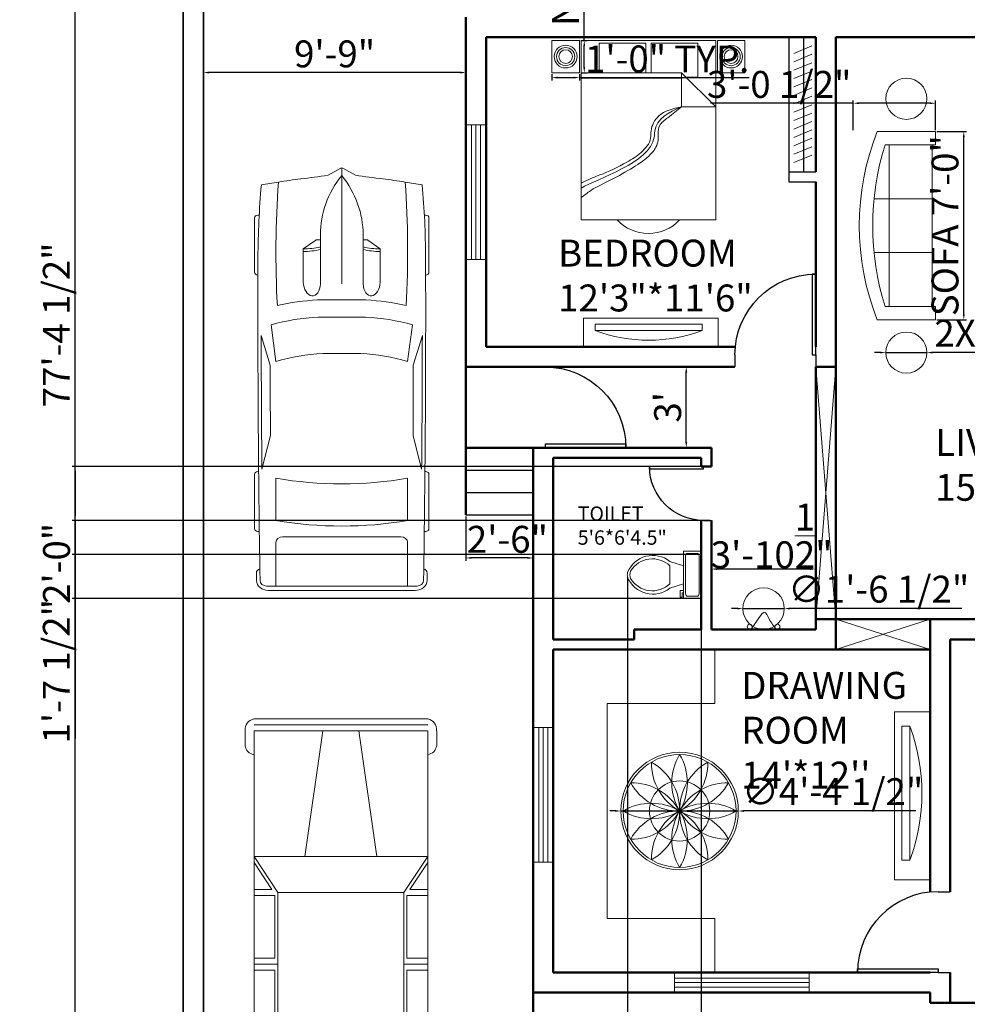
# Model space of a CAD drawing. Units: inches. Extents: x 6286 to 7213, y 5725 to 6776.
# Tile 2 of 5: x 6286 to 6709, y 5946 to 6385. Entities that reach past the tile are written whole.
import ezdxf

# ---------------------------------------------------------------- set-up
doc = ezdxf.new("R2010")
doc.units = ezdxf.units.IN
for name, color, linetype, lineweight in [('A-ANNO-DIMS', 2, 'Continuous', 18), ('A-AREA-IDEN', 7, 'Continuous', 25), ('A-DOOR', 3, 'Continuous', 25), ('A-FLOR-CASE', 8, 'Continuous', 25), ('A-FLOR-CASE-PATT', 252, 'Continuous', 13), ('A-FLOR-STRS', 7, 'Continuous', 25), ('A-FURN', 8, 'Continuous', 18), ('A-GLAZ', 4, 'Continuous', 18), ('A-WALL', 7, 'Continuous', 50), ('A-WALL-OPEN', 7, 'Continuous', 18), ('C-PKNG-VEHI', 8, 'Continuous', 13), ('C-PROP', 7, 'Continuous', 35), ('P-FLOR-FIXT', 9, 'Continuous', 18)]:
    doc.layers.add(name, color=color, linetype=linetype, lineweight=lineweight)
doc.styles.get("Standard").update_dxf_attribs({"font": 'arial.ttf'})
doc.dimstyles.new('ISO-25', dxfattribs={"dimtxt": 12, "dimasz": 2.5, "dimexe": 1.25, "dimexo": 0.625, "dimtad": 1, "dimdec": 1, "dimlunit": 4, "dimtxsty": 'Standard', "dimcen": 2.5, "dimadec": 0, "dimazin": 0, "dimtfac": 1, "dimtdec": 1, "dimtmove": 0, "dimatfit": 3, "dimfxl": 1, "dimarcsym": 0})

# ---------------------------------------------------------------- blocks, each defined once
blk = doc.blocks.new('*U2')
for p, q in [((0, 0), (0, -6)), ((40, 0), (40, -6))]:
    blk.add_line(p, q)
blk.add_lwpolyline([(0, 0), (0, 40), (1.75, 40), (1.75, 0)], close=True)
blk.add_arc((0, 0), 40, 0, 90)
blk = doc.blocks.new('*U10')
for p, q in [((9.5, -6), (9.5, -2)), ((-10, -8.5), (-8, -8.5)), ((-10, -9.5), (-10, -8.5)), ((-8, -8.5), (-8, -8)), ((-7, -8), (-7, -9.5)), ((-4, -8), (-6, -14)), ((4, -8), (6, -14)), ((-7, -9.5), (-10, -9.5)), ((4, -14), (-4, -14))]:
    blk.add_line(p, q)
blk.add_lwpolyline([(10.5, -8), (10.5, 0), (-10.5, 0), (-10.5, -8)], close=True)
for points in [[(-9.5, -2), (-9.5, -6)], [(8.5, -1), (-8.5, -1)], [(-8.5, -7), (8.5, -7)]]:
    blk.add_lwpolyline(points)
for centre, radius, start, end in [((-8.62, -1.88), 0.884, 81.8699, 188.1301), ((8.62, -1.88), 0.884, 351.8699, 98.1301), ((-8.62, -6.12), 0.884, 171.8699, 278.1301), ((8.62, -6.12), 0.884, 261.8699, 8.1301), ((3.52, -21.58), 12.17, 141.4691, 247.9714), ((4.2, -21.82), 11.33, 136.3677, 238.9468), ((-3.52, -21.58), 12.17, 292.0284, 38.5307), ((-4.2, -21.82), 11.33, 301.053, 43.6321), ((0, -27.88), 4, 245.7318, 294.2682), ((0, -29), 4, 254.8605, 285.1395)]:
    blk.add_arc(centre, radius, start, end)
blk = doc.blocks.new('Sofa - Roundback 7 ft.')
for p, q in [((-12.00002, -32.4421), (-12.00003, -6.5971)), ((11.99997, -32.4421), (11.99998, -6.5971)), ((-36.000027, -34), (-36.000027, -11.4696)), ((35.99998, -34), (35.99998, -11.4696)), ((-35.999844, -13.3819), (35.9998, -13.3819)), ((-36.000027, -32.4421), (35.99998, -32.4421))]:
    blk.add_line(p, q)
for points in [[(-36.000027, -34), (-42.000027, -34), (-42.000027, -8)], [(41.99998, -8), (41.99998, -34), (35.99998, -34)]]:
    blk.add_lwpolyline(points)
for centre, radius, start, end in [((0, -114.25), 114.25, 68.43141, 111.5686), ((-0.00001, -127.1968), 121.1968, 72.72033, 107.2797)]:
    blk.add_arc(centre, radius, start, end)
blk = doc.blocks.new('*D13')
at = {"layer": 'A-ANNO-DIMS', "color": 0, "lineweight": -2, "transparency": 16777216}
for p, q in [((6593.8, 6230.26), (6581.95, 6230.26)), ((6583.2, 6196.76), (6583.2, 6227.76)), ((6593.8, 6194.26), (6581.95, 6194.26))]:
    blk.add_line(p, q, dxfattribs=at)
at = {"layer": 'A-ANNO-DIMS', "color": 0, "lineweight": 100, "transparency": 16777216}
for points in [[(6582.79, 6227.76), (6583.62, 6227.76), (6583.2, 6230.26)], [(6582.79, 6196.76), (6583.62, 6196.76), (6583.2, 6194.26)]]:
    blk.add_solid(points, dxfattribs=at)
at = {"layer": 'Defpoints', "color": 0, "lineweight": 100, "transparency": 16777216}
for p in [(6583.2, 6230.26), (6594.42, 6230.26), (6594.42, 6194.26)]:
    blk.add_point(p, dxfattribs=at)
at = {"layer": 'A-ANNO-DIMS', "color": 0, "transparency": 16777216, "insert": (6576.45, 6212.26), "char_height": 12, "attachment_point": 5, "rotation": 90}
blk.add_mtext("3'", dxfattribs=at)
blk = doc.blocks.new('*D14')
at = {"layer": 'A-ANNO-DIMS', "color": 0, "lineweight": -2, "transparency": 16777216}
for p, q in [((6484.92, 6163.64), (6484.92, 6143.83)), ((6514.92, 6163.64), (6514.92, 6143.83)), ((6512.42, 6145.08), (6487.42, 6145.08))]:
    blk.add_line(p, q, dxfattribs=at)
at = {"layer": 'A-ANNO-DIMS', "color": 0, "lineweight": 100, "transparency": 16777216}
for points in [[(6487.42, 6145.5), (6487.42, 6144.67), (6484.92, 6145.08)], [(6512.42, 6145.5), (6512.42, 6144.67), (6514.92, 6145.08)]]:
    blk.add_solid(points, dxfattribs=at)
at = {"layer": 'Defpoints', "color": 0, "lineweight": 100, "transparency": 16777216}
for p in [(6484.92, 6164.26), (6514.92, 6164.26), (6484.92, 6145.08)]:
    blk.add_point(p, dxfattribs=at)
at = {"layer": 'A-ANNO-DIMS', "color": 0, "transparency": 16777216, "insert": (6503.46, 6151.84), "char_height": 12, "attachment_point": 5}
blk.add_mtext('2\'-6"', dxfattribs=at)
blk = doc.blocks.new('*D15')
at = {"layer": 'A-ANNO-DIMS', "color": 0, "lineweight": -2, "transparency": 16777216}
for p, q in [((6594.42, 6113.89), (6594.42, 6141.38)), ((6638.42, 6140.13), (6596.92, 6140.13)), ((6640.92, 6113.89), (6640.92, 6141.38))]:
    blk.add_line(p, q, dxfattribs=at)
at = {"layer": 'A-ANNO-DIMS', "color": 0, "lineweight": 100, "transparency": 16777216}
for points in [[(6596.92, 6140.55), (6596.92, 6139.71), (6594.42, 6140.13)], [(6638.42, 6140.55), (6638.42, 6139.71), (6640.92, 6140.13)]]:
    blk.add_solid(points, dxfattribs=at)
at = {"layer": 'Defpoints', "color": 0, "lineweight": 100, "transparency": 16777216}
for p in [(6594.42, 6140.13), (6594.42, 6113.26), (6640.92, 6113.26)]:
    blk.add_point(p, dxfattribs=at)
at = {"layer": 'A-ANNO-DIMS', "color": 0, "transparency": 16777216, "insert": (6621.27, 6154.91), "char_height": 12, "attachment_point": 5}
blk.add_mtext('3\'-10{\\H1x;\\S1/2;}"', dxfattribs=at)
blk = doc.blocks.new('*D25')
at = {"layer": 'A-ANNO-DIMS', "color": 0, "lineweight": -2, "transparency": 16777216}
for p, q in [((6367.92, 6385.64), (6367.92, 6360.28)), ((6484.92, 6385.64), (6484.92, 6360.28)), ((6482.42, 6361.53), (6370.42, 6361.53))]:
    blk.add_line(p, q, dxfattribs=at)
at = {"layer": 'A-ANNO-DIMS', "color": 0, "lineweight": 100, "transparency": 16777216}
for points in [[(6370.42, 6361.95), (6370.42, 6361.12), (6367.92, 6361.53)], [(6482.42, 6361.95), (6482.42, 6361.12), (6484.92, 6361.53)]]:
    blk.add_solid(points, dxfattribs=at)
at = {"layer": 'Defpoints', "color": 0, "lineweight": 100, "transparency": 16777216}
for p in [(6367.92, 6386.26), (6484.92, 6386.26), (6367.92, 6361.53)]:
    blk.add_point(p, dxfattribs=at)
at = {"layer": 'A-ANNO-DIMS', "color": 0, "transparency": 16777216, "insert": (6426.42, 6368.29), "char_height": 12, "attachment_point": 5}
blk.add_mtext('9\'-9"', dxfattribs=at)
blk = doc.blocks.new('*U27')
for p, q in [((21.1, 37.41), (21.1, 36.83)), ((46.55, 38.89), (22.35, 38.89)), ((47.8, 37.39), (47.8, 37.41)), ((87.99, 31.87), (74.76, 35.92)), ((134.31, 35.6), (119.29, 31.78)), ((135.45, 37.07), (135.45, 37.41)), ((136.7, 38.89), (160.9, 38.89)), ((162.15, 37.41), (162.15, 36.77)), ((70.03, 31.54), (86.41, 29.35)), ((186.47, -33.5), (186.47, 33.5)), ((188.4, -32.76), (188.4, 32.76)), ((138.42, 29.35), (157.25, 29.35)), ((164.52, 26.39), (164.52, -26.39)), ((186.47, 29.35), (167.01, 29.35)), ((32.27, 11.63), (36.13, 17.17)), ((36.13, 17.17), (50.94, 17.17)), ((29.77, 9.51), (51.68, 9.51)), ((32.12, 9.51), (32.12, 11.15)), ((58.92, -10.77), (58.92, 10.77)), ((66.55, -10.53), (66.55, 10.53)), ((186.47, -10.53), (186.47, 10.53)), ((3.27, 6.13), (0.1, 0.41)), ((82.74, 8.5), (82.74, -8.5)), ((0, 0), (51.68, 0)), ((0.1, -0.41), (3.27, -6.13)), ((29.77, -9.51), (51.68, -9.51)), ((32.12, -9.51), (32.12, -11.15)), ((32.27, -11.63), (36.13, -17.17)), ((36.13, -17.17), (50.94, -17.17)), ((86.41, -29.35), (70.03, -31.54)), ((157.25, -29.35), (138.42, -29.35)), ((167.01, -29.35), (186.47, -29.35)), ((87.99, -31.87), (74.76, -35.92)), ((134.31, -35.6), (119.29, -31.78)), ((21.1, -37.41), (21.1, -36.83)), ((46.55, -38.89), (22.35, -38.89)), ((47.8, -37.39), (47.8, -37.41)), ((135.45, -37.07), (135.45, -37.41)), ((136.7, -38.89), (160.9, -38.89)), ((162.15, -37.41), (162.15, -36.77))]:
    blk.add_line(p, q)
for centre, major_axis, ratio, start_param, end_param in [((266.03, -27.52), (0, 313.31), 0.842304, 1.367076, 1.39176), ((41.19, -490.86), (0, 528.23), 0.842304, 0.00281, 0.075598), ((22.35, 37.41), (0, -1.48), 0.842304, 3.141593, 4.712389), ((64.48, -10555.62), (0, 10593.03), 0.842304, -0.013397, 0.002797), ((46.55, 37.41), (0, 1.48), 0.842304, -1.570796, 0), ((64.48, -10555.62), (0, -10591.55), 0.842304, 3.133765, 3.140441), ((136.7, 37.41), (0, -1.48), 0.842304, 3.141593, 4.712389), ((160.9, 37.41), (0, 1.48), 0.842304, -1.570796, 0), ((180.63, 35.84), (0, 2.22), 0.842304, -0.013017, 1.249894), ((64.48, -10556.36), (0, 10595.31), 0.842304, -0.013397, -0.013017), ((183.98, 33.5), (0, -2.96), 0.842304, 1.570796, 3.128196), ((183.98, 32.76), (0, -5.25), 0.842304, 1.570796, 3.128196), ((135.29, 5.39), (0, 81.77), 0.842304, 1.245306, 1.50788), ((95.79, -3666.35), (0, -3698.24), 0.842304, 3.134049, 3.144098), ((259.18, -27.52), (0, -305.3), 0.842304, 4.528606, 4.561838), ((37.47, -593.96), (0, -623.33), 0.842304, 3.096046, 3.200911), ((134.4, 5.39), (0, -89.78), 0.842304, 4.449482, 4.652344), ((149.6, 2.8), (0, -79.58), 0.842304, 4.372215, 4.640744), ((17.08, 0), (0, 147.02), 0.842304, 4.511394, 4.913384), ((35.91, 0), (0, 147.02), 0.842304, 4.511394, 4.913384), ((167.01, 26.39), (0, 2.96), 0.842304, 0, 1.570796), ((-204.49, 52.4), (0, -250.96), 0.842304, 1.385369, 1.434372), ((13.04, 17.01), (0, 27.42), 0.842304, 4.435146, 4.718221), ((14.2, 17.01), (0, 27.42), 0.842304, 4.435146, 4.718221), ((50.79, 13.34), (6.34, -0.36), 0.603834, -1.395552, 1.581315), ((29.77, -46.66), (0, 56.17), 0.842304, 0, 0.590319), ((32.75, 11.15), (0, 0.74), 0.842304, 0.879714, 1.570796), ((0.62, 0), (0, -0.74), 0.842304, 4.131459, 5.293319), ((29.77, 46.66), (0, 56.17), 0.842304, 2.551274, 3.141593), ((-204.49, -52.4), (0, 250.96), 0.842304, -1.434372, -1.385369), ((149.6, -2.8), (0, -79.58), 0.842304, -1.499151, -1.230623), ((32.75, -11.15), (0, -0.74), 0.842304, 4.712389, 5.403472), ((13.04, -17.01), (0, -27.42), 0.842304, 1.564964, 1.848039), ((14.2, -17.01), (0, -27.42), 0.842304, 1.564964, 1.848039), ((134.4, -5.39), (0, -89.78), 0.842304, -1.510751, -1.307889), ((135.29, -5.39), (0, -81.77), 0.842304, -1.50788, -1.245306), ((259.18, 27.52), (0, 305.3), 0.842304, 1.721348, 1.754579), ((266.03, 27.52), (0, 313.31), 0.842304, 1.749832, 1.774517), ((37.47, 593.96), (0, -623.33), 0.842304, -0.059319, 0.045547), ((167.01, -26.39), (0, -2.96), 0.842304, 4.712389, 6.283185), ((95.79, 3666.35), (0, -3698.24), 0.842304, -0.002505, 0.007544), ((183.98, -33.5), (0, 2.96), 0.842304, 3.15499, 4.712389), ((183.98, -32.76), (0, -5.25), 0.842304, 0.013397, 1.570796), ((41.19, 490.86), (0, -528.23), 0.842304, -0.075598, -0.00281), ((22.35, -37.41), (0, 1.48), 0.842304, 1.570796, 3.141593), ((64.48, 10555.62), (0, 10593.03), 0.842304, 3.138796, 3.15499), ((46.55, -37.41), (0, -1.48), 0.842304, 0, 1.570796), ((64.48, 10555.62), (0, -10591.55), 0.842304, 0.001152, 0.007828), ((136.7, -37.41), (0, -1.48), 0.842304, -1.570796, 0), ((160.9, -37.41), (0, 1.48), 0.842304, 3.141593, 4.712389), ((180.63, -35.84), (0, -2.22), 0.842304, -1.249894, 0.013017), ((64.48, 10556.36), (0, 10595.31), 0.842304, 3.15461, 3.15499)]:
    blk.add_ellipse(centre, major_axis=major_axis, ratio=ratio, start_param=start_param, end_param=end_param)
at = {"extrusion": (0, 0, -1)}
blk.add_ellipse((50.79, -13.34), major_axis=(6.34, 0.36), ratio=0.603834, start_param=-1.395552, end_param=1.581315, dxfattribs=at)
blk = doc.blocks.new('*U28')
for p, q in [((5.44, 42.31), (12.12, 42.31)), ((189.69, 42.31), (183.01, 42.31)), ((0.1, -0.41), (0.1, 38.35)), ((2.77, -0.41), (2.77, 38.31)), ((5.44, -0.41), (5.44, 38.24)), ((5.45, 38.31), (16.12, 38.31)), ((16.12, 38.31), (180.34, 38.31)), ((61.52, -0.41), (61.52, 38.31)), ((61.52, 38.31), (77.54, 27.62)), ((64.19, 38.31), (76.2, 30.29)), ((76.2, 30.29), (76.2, 38.31)), ((78.87, 38.31), (78.87, 28.96)), ((106.91, 28.96), (106.91, 38.31)), ((109.58, 27.62), (109.58, 38.31)), ((112.25, 38.31), (112.25, 28.96)), ((140.29, 28.96), (140.29, 38.31)), ((141.62, 27.62), (149.64, 38.31)), ((149.64, -0.41), (149.64, 38.31)), ((189.69, 38.31), (179.01, 38.31)), ((189.69, -0.41), (189.69, 38.24)), ((192.36, -0.41), (192.36, 38.31)), ((195.03, -0.41), (195.03, 38.35)), ((77.54, 27.62), (141.62, 27.62)), ((77.54, -0.41), (77.54, 27.62)), ((78.87, 28.96), (106.91, 28.96)), ((112.25, 28.96), (140.29, 28.96)), ((141.62, -0.41), (141.62, 27.62)), ((5.44, 7.6), (61.52, 15.61)), ((0.1, -0.42), (0.1, -39.18)), ((2.77, -0.41), (2.77, -39.13)), ((5.44, -0.42), (5.44, -39.07)), ((61.52, -0.41), (61.52, -39.13)), ((77.54, -0.41), (77.54, -28.45)), ((141.62, -0.41), (141.62, -28.45)), ((149.64, -0.41), (149.64, -39.13)), ((189.69, -0.42), (189.69, -39.07)), ((192.36, -0.41), (192.36, -39.13)), ((195.03, -0.42), (195.03, -39.18)), ((5.44, -8.42), (61.52, -16.43)), ((61.52, -39.13), (77.54, -28.45)), ((77.54, -28.45), (141.62, -28.45)), ((78.87, -39.13), (78.87, -29.79)), ((78.87, -29.79), (106.91, -29.79)), ((106.91, -29.79), (106.91, -39.13)), ((109.58, -28.45), (109.58, -39.13)), ((112.25, -29.79), (140.29, -29.79)), ((112.25, -39.13), (112.25, -29.79)), ((140.29, -29.79), (140.29, -39.13)), ((141.62, -28.45), (149.64, -39.13)), ((64.19, -39.13), (76.2, -31.12)), ((76.2, -31.12), (76.2, -39.13)), ((5.45, -39.13), (16.12, -39.13)), ((16.12, -39.13), (180.34, -39.13)), ((189.69, -39.13), (179.01, -39.13)), ((5.44, -43.14), (12.12, -43.14)), ((189.69, -43.14), (183.01, -43.14))]:
    blk.add_line(p, q)
for centre, radius, start, end in [((5.06, 37.26), 5.06, 85.6455, 168.0943), ((11.45, 37.64), 4.72, 8.1301, 81.87), ((183.68, 37.64), 4.72, 98.13, 171.8699), ((190.07, 37.26), 5.06, 11.9057, 94.3545), ((5.06, -38.09), 5.06, 191.9057, 274.3545), ((11.45, -38.46), 4.72, 278.13, 351.8699), ((183.68, -38.46), 4.72, 188.1301, 261.87), ((190.07, -38.09), 5.06, 265.6455, 348.0943)]:
    blk.add_arc(centre, radius, start, end)
blk = doc.blocks.new('WIN-60IN')
for p, q in [((0, 9), (0, 0)), ((60, 0), (60, 9)), ((60, 6.5), (0, 6.5)), ((60, 4.5), (0, 4.5)), ((60, 2.5), (0, 2.5))]:
    blk.add_line(p, q)
blk = doc.blocks.new('NIGHTSTAND-LAMP')
blk.add_lwpolyline([(12.23, 14.4), (0, 14.4), (0, 0), (12.23, 0)], close=True)
for radius in [5.06, 4.06, 3.06]:
    blk.add_circle((6.12, 7.2), radius)
blk = doc.blocks.new('TV-CONSOLE-60IN')
for points in [[(0, 12.71), (60, 12.71), (60, 0), (0, 0)], [(5.19, 10.13), (52.94, 10.13), (52.94, 7.18), (5.19, 7.18)]]:
    blk.add_lwpolyline(points, close=True)
blk.add_arc((29.07, 71.71), 68.81, 249.6947, 290.3053)
blk = doc.blocks.new('Bed - Queen')
for p, q in [((0, -80.00003), (0, 0)), ((0, 0), (59.99999, 0)), ((59.99999, 0), (59.99999, -80.00003)), ((7.99999, -1.2), (28.79998, -1.2)), ((7.99999, -14.4), (7.99999, -1.2)), ((28.79998, -1.2), (28.79998, -14.4)), ((31.19999, -1.2), (51.99999, -1.2)), ((31.19999, -14.4), (31.19999, -1.2)), ((51.99999, -1.2), (51.99999, -16.4)), ((0, -14.4), (44.8, -14.4)), ((44.8, -16.8), (0, -16.8)), ((59.99999, -29.6), (44.8, -14.4)), ((44.8, -14.4), (44.8, -29.6)), ((51.99999, -16.4), (46.79936, -16.4)), ((44.8, -29.6), (59.99999, -29.6)), ((59.99999, -80.00003), (0, -80.00003))]:
    blk.add_line(p, q)
blk = doc.blocks.new('BED-QUEEN-DRESSED')
blk.add_arc((30, 18.96), 18.96, 222.7518, 317.2482)
for points, knots in [([(44.8, 56.49), (39.19, 53.96), (32.77, 51.07), (32.71, 32.08), (7.2, 24.53), (0, 20.27)], [0, 0, 0, 0, 16.08431, 18.417841, 48.068097, 48.068097, 48.068097, 48.068097]), ([(44.8, 56.49), (41.02, 55.65), (34.77, 54.26), (30.9, 47.2), (31.38, 41.03), (26.76, 35.63), (19.36, 31.03), (9.68, 26.38), (4.48, 24.69), (0, 22.46)], [0, 0, 0, 0, 11.066231, 18.341473, 21.645482, 29.256421, 37.126455, 49.94498, 57.001864, 57.001864, 57.001864, 57.001864]), ([(44.8, 56.49), (42.82, 54.88), (39.55, 52.2), (33.5, 47.94), (35.23, 40.79), (30.55, 34.13), (23.14, 29.37), (13.11, 23.54), (6.2, 20.75), (1.43, 17.09), (0, 16.03)], [0, 0, 0, 0, 7.83924, 12.978287, 20.287315, 26.568624, 36.127852, 46.548326, 57.45004, 62.118815, 62.118815, 62.118815, 62.118815])]:
    blk.add_open_spline(points, degree=3, knots=knots)
blk.add_blockref('Bed - Queen', (0, 86.09))
blk = doc.blocks.new('WARDROBE-RETURN-RAIL')
for p, q in [((0, 64.5), (0, 0)), ((6.49, 64.5), (6.49, 4.5)), ((0, 4.5), (12, 4.5)), ((0, 0), (12, 0))]:
    blk.add_line(p, q)
blk = doc.blocks.new('*D43')
at = {"layer": 'A-ANNO-DIMS', "color": 0, "lineweight": -2, "transparency": 16777216}
for p, q in [((6537.72, 6375.84), (6537.72, 6593.74)), ((6536.18, 6375.84), (6538.97, 6375.84)), ((6537.72, 6363.94), (6537.72, 6373.34)), ((6536.18, 6361.44), (6538.97, 6361.44))]:
    blk.add_line(p, q, dxfattribs=at)
at = {"layer": 'A-ANNO-DIMS', "color": 0, "lineweight": 100, "transparency": 16777216}
for points in [[(6537.3, 6373.34), (6538.13, 6373.34), (6537.72, 6375.84)], [(6537.3, 6363.94), (6538.13, 6363.94), (6537.72, 6361.44)]]:
    blk.add_solid(points, dxfattribs=at)
at = {"layer": 'Defpoints', "color": 0, "lineweight": 100, "transparency": 16777216}
for p in [(6535.56, 6375.84), (6537.72, 6375.84), (6535.56, 6361.44)]:
    blk.add_point(p, dxfattribs=at)
at = {"layer": 'A-ANNO-DIMS', "color": 0, "transparency": 16777216, "insert": (6530.89, 6486.04), "char_height": 12, "attachment_point": 5, "rotation": 90}
blk.add_mtext('NIGHTSTAND 1\'-2 1/2" TYP.', dxfattribs=at)
blk = doc.blocks.new('*D44')
at = {"layer": 'A-ANNO-DIMS', "color": 0, "lineweight": -2, "transparency": 16777216}
for p, q in [((6523.32, 6360.81), (6523.32, 6358.03)), ((6525.82, 6359.28), (6533.06, 6359.28)), ((6535.56, 6360.81), (6535.56, 6358.03)), ((6535.56, 6359.28), (6611.32, 6359.28))]:
    blk.add_line(p, q, dxfattribs=at)
at = {"layer": 'A-ANNO-DIMS', "color": 0, "lineweight": 100, "transparency": 16777216}
for points in [[(6525.82, 6359.69), (6525.82, 6358.86), (6523.32, 6359.28)], [(6533.06, 6359.69), (6533.06, 6358.86), (6535.56, 6359.28)]]:
    blk.add_solid(points, dxfattribs=at)
at = {"layer": 'Defpoints', "color": 0, "lineweight": 100, "transparency": 16777216}
for p in [(6523.32, 6361.44), (6535.56, 6361.44), (6535.56, 6359.28)]:
    blk.add_point(p, dxfattribs=at)
at = {"layer": 'A-ANNO-DIMS', "color": 0, "transparency": 16777216, "insert": (6574.69, 6366.03), "char_height": 12, "attachment_point": 5}
blk.add_mtext('1\'-0" TYP.', dxfattribs=at)
blk = doc.blocks.new('*D53')
at = {"layer": 'A-ANNO-DIMS', "color": 0, "lineweight": -2, "transparency": 16777216}
for p, q in [((6694.98, 6335.25), (6708.2, 6335.25)), ((6706.95, 6253.75), (6706.95, 6332.75)), ((6694.98, 6251.25), (6708.2, 6251.25))]:
    blk.add_line(p, q, dxfattribs=at)
at = {"layer": 'A-ANNO-DIMS', "color": 0, "lineweight": 100, "transparency": 16777216}
for points in [[(6706.54, 6332.75), (6707.37, 6332.75), (6706.95, 6335.25)], [(6706.54, 6253.75), (6707.37, 6253.75), (6706.95, 6251.25)]]:
    blk.add_solid(points, dxfattribs=at)
at = {"layer": 'Defpoints', "color": 0, "lineweight": 100, "transparency": 16777216}
for p in [(6694.35, 6335.25), (6706.95, 6335.25), (6694.35, 6251.25)]:
    blk.add_point(p, dxfattribs=at)
at = {"layer": 'A-ANNO-DIMS', "color": 0, "transparency": 16777216, "insert": (6700.12, 6293.25), "char_height": 12, "attachment_point": 5, "rotation": 90}
blk.add_mtext('SOFA 7\'-0"', dxfattribs=at)
blk = doc.blocks.new('*D54')
at = {"layer": 'A-ANNO-DIMS', "color": 0, "lineweight": -2, "transparency": 16777216}
for p, q in [((6657.69, 6335.87), (6657.69, 6349.1)), ((6694.35, 6335.87), (6694.35, 6349.1)), ((6657.69, 6347.85), (6594.08, 6347.85)), ((6691.85, 6347.85), (6660.19, 6347.85))]:
    blk.add_line(p, q, dxfattribs=at)
at = {"layer": 'A-ANNO-DIMS', "color": 0, "lineweight": 100, "transparency": 16777216}
for points in [[(6660.19, 6348.26), (6660.19, 6347.43), (6657.69, 6347.85)], [(6691.85, 6348.26), (6691.85, 6347.43), (6694.35, 6347.85)]]:
    blk.add_solid(points, dxfattribs=at)
at = {"layer": 'Defpoints', "color": 0, "lineweight": 100, "transparency": 16777216}
for p in [(6657.69, 6347.85), (6657.69, 6335.25), (6694.35, 6335.25)]:
    blk.add_point(p, dxfattribs=at)
at = {"layer": 'A-ANNO-DIMS', "color": 0, "transparency": 16777216, "insert": (6624.64, 6354.68), "char_height": 12, "attachment_point": 5}
blk.add_mtext('3\'-0 1/2"', dxfattribs=at)
blk = doc.blocks.new('*D56')
at = {"layer": 'A-ANNO-DIMS', "color": 0, "lineweight": -2, "transparency": 16777216}
for p, q in [((6358.3, 6713.26), (6309.47, 6713.26)), ((6310.72, 5787.26), (6310.72, 6710.76)), ((6358.3, 5784.76), (6309.47, 5784.76))]:
    blk.add_line(p, q, dxfattribs=at)
at = {"layer": 'A-ANNO-DIMS', "color": 0, "lineweight": 100, "transparency": 16777216}
for points in [[(6310.31, 6710.76), (6311.14, 6710.76), (6310.72, 6713.26)], [(6310.31, 5787.26), (6311.14, 5787.26), (6310.72, 5784.76)]]:
    blk.add_solid(points, dxfattribs=at)
at = {"layer": 'Defpoints', "color": 0, "lineweight": 100, "transparency": 16777216}
for p in [(6310.72, 6713.26), (6358.92, 6713.26), (6358.92, 5784.76)]:
    blk.add_point(p, dxfattribs=at)
at = {"layer": 'A-ANNO-DIMS', "color": 0, "transparency": 16777216, "insert": (6303.89, 6249.01), "char_height": 12, "attachment_point": 5, "rotation": 90}
blk.add_mtext('77\'-4 1/2"', dxfattribs=at)
blk = doc.blocks.new('*D68')
at = {"layer": 'A-ANNO-DIMS', "color": 0, "lineweight": -2, "transparency": 16777216}
for p, q in [((6593.8, 6185.85), (6309.47, 6185.85)), ((6310.72, 6183.35), (6310.72, 6164.35)), ((6593.8, 6161.85), (6309.47, 6161.85)), ((6310.72, 6161.85), (6310.72, 6126))]:
    blk.add_line(p, q, dxfattribs=at)
at = {"layer": 'A-ANNO-DIMS', "color": 0, "lineweight": 100, "transparency": 16777216}
for points in [[(6310.31, 6183.35), (6311.14, 6183.35), (6310.72, 6185.85)], [(6310.31, 6164.35), (6311.14, 6164.35), (6310.72, 6161.85)]]:
    blk.add_solid(points, dxfattribs=at)
at = {"layer": 'Defpoints', "color": 0, "lineweight": 100, "transparency": 16777216}
for p in [(6594.42, 6185.85), (6310.72, 6161.85), (6594.42, 6161.85)]:
    blk.add_point(p, dxfattribs=at)
at = {"layer": 'A-ANNO-DIMS', "color": 0, "transparency": 16777216, "insert": (6303.97, 6142.67), "char_height": 12, "attachment_point": 5, "rotation": 90}
blk.add_mtext('2\'-0"', dxfattribs=at)
blk = doc.blocks.new('*D69')
at = {"layer": 'A-ANNO-DIMS', "color": 0, "lineweight": -2, "transparency": 16777216}
for p, q in [((6589.3, 6146.57), (6309.47, 6146.57)), ((6310.72, 6144.07), (6310.72, 6129.57)), ((6589.3, 6127.07), (6309.47, 6127.07)), ((6310.72, 6127.07), (6310.72, 6064.58))]:
    blk.add_line(p, q, dxfattribs=at)
at = {"layer": 'A-ANNO-DIMS', "color": 0, "lineweight": 100, "transparency": 16777216}
for points in [[(6310.31, 6144.07), (6311.14, 6144.07), (6310.72, 6146.57)], [(6310.31, 6129.57), (6311.14, 6129.57), (6310.72, 6127.07)]]:
    blk.add_solid(points, dxfattribs=at)
at = {"layer": 'Defpoints', "color": 0, "lineweight": 100, "transparency": 16777216}
for p in [(6589.92, 6146.57), (6310.72, 6127.07), (6589.92, 6127.07)]:
    blk.add_point(p, dxfattribs=at)
at = {"layer": 'A-ANNO-DIMS', "color": 0, "transparency": 16777216, "insert": (6303.89, 6094.57), "char_height": 12, "attachment_point": 5, "rotation": 90}
blk.add_mtext('1\'-7 1/2"', dxfattribs=at)
blk = doc.blocks.new('*D70')
at = {"layer": 'A-ANNO-DIMS', "color": 0, "lineweight": -2, "transparency": 16777216}
for p, q in [((6556.96, 6136.41), (6556.96, 5735.31)), ((6589.92, 6126.44), (6589.92, 5735.31)), ((6559.46, 5736.56), (6587.42, 5736.56)), ((6589.92, 5736.56), (6625.78, 5736.56))]:
    blk.add_line(p, q, dxfattribs=at)
at = {"layer": 'A-ANNO-DIMS', "color": 0, "lineweight": 100, "transparency": 16777216}
for points in [[(6559.46, 5736.98), (6559.46, 5736.15), (6556.96, 5736.56)], [(6587.42, 5736.98), (6587.42, 5736.15), (6589.92, 5736.56)]]:
    blk.add_solid(points, dxfattribs=at)
at = {"layer": 'Defpoints', "color": 0, "lineweight": 100, "transparency": 16777216}
for p in [(6556.96, 6137.04), (6589.92, 6127.07), (6589.92, 5736.56)]:
    blk.add_point(p, dxfattribs=at)
at = {"layer": 'A-ANNO-DIMS', "color": 0, "transparency": 16777216, "insert": (6609.1, 5743.32), "char_height": 12, "attachment_point": 5}
blk.add_mtext('2\'-9"', dxfattribs=at)
blk = doc.blocks.new('*D75')
at = {"layer": 'A-ANNO-DIMS', "color": 0, "lineweight": -2, "transparency": 16777216}
for p, q in [((6669.69, 6236.66), (6667.19, 6236.66)), ((6672.19, 6236.66), (6690.52, 6236.66)), ((6795.04, 6236.67), (6693.02, 6236.66))]:
    blk.add_line(p, q, dxfattribs=at)
at = {"layer": 'A-ANNO-DIMS', "color": 0, "lineweight": 100, "transparency": 16777216}
for points in [[(6669.69, 6237.08), (6669.69, 6236.25), (6672.19, 6236.66)], [(6693.02, 6237.08), (6693.02, 6236.25), (6690.52, 6236.66)]]:
    blk.add_solid(points, dxfattribs=at)
at = {"layer": 'Defpoints', "color": 0, "lineweight": 100, "transparency": 16777216}
for p in [(6672.19, 6236.66), (6690.52, 6236.66)]:
    blk.add_point(p, dxfattribs=at)
at = {"layer": 'A-ANNO-DIMS', "color": 0, "transparency": 16777216, "insert": (6745.28, 6243.75), "char_height": 12, "attachment_point": 5, "rotation": 0.0013}
blk.add_mtext('2X ∅1\'-6 1/2"', dxfattribs=at)
blk = doc.blocks.new('*D77')
at = {"layer": 'A-ANNO-DIMS', "color": 0, "lineweight": -2, "transparency": 16777216}
for p, q in [((6551.56, 6032.26), (6549.06, 6032.26)), ((6554.06, 6032.26), (6606.42, 6032.26)), ((6685.59, 6032.26), (6608.92, 6032.26))]:
    blk.add_line(p, q, dxfattribs=at)
at = {"layer": 'A-ANNO-DIMS', "color": 0, "lineweight": 100, "transparency": 16777216}
for points in [[(6551.56, 6032.68), (6551.56, 6031.85), (6554.06, 6032.26)], [(6608.92, 6032.68), (6608.92, 6031.85), (6606.42, 6032.26)]]:
    blk.add_solid(points, dxfattribs=at)
at = {"layer": 'Defpoints', "color": 0, "lineweight": 100, "transparency": 16777216}
for p in [(6554.06, 6032.26), (6606.42, 6032.26)]:
    blk.add_point(p, dxfattribs=at)
at = {"layer": 'A-ANNO-DIMS', "color": 0, "transparency": 16777216, "insert": (6648.51, 6039.35), "char_height": 12, "attachment_point": 5, "rotation": 359.9989}
blk.add_mtext('∅4\'-4 1/2"', dxfattribs=at)
blk = doc.blocks.new('*D78')
at = {"layer": 'A-ANNO-DIMS', "color": 0, "lineweight": -2, "transparency": 16777216}
for p, q in [((6605.92, 6122.52), (6603.42, 6122.52)), ((6608.42, 6122.52), (6626.93, 6122.52)), ((6706.09, 6122.51), (6629.43, 6122.52))]:
    blk.add_line(p, q, dxfattribs=at)
at = {"layer": 'A-ANNO-DIMS', "color": 0, "lineweight": 100, "transparency": 16777216}
for points in [[(6605.92, 6122.93), (6605.92, 6122.1), (6608.42, 6122.52)], [(6629.43, 6122.93), (6629.43, 6122.1), (6626.93, 6122.52)]]:
    blk.add_solid(points, dxfattribs=at)
at = {"layer": 'Defpoints', "color": 0, "lineweight": 100, "transparency": 16777216}
for p in [(6608.42, 6122.52), (6626.93, 6122.52)]:
    blk.add_point(p, dxfattribs=at)
at = {"layer": 'A-ANNO-DIMS', "color": 0, "transparency": 16777216, "insert": (6669.01, 6129.6), "char_height": 12, "attachment_point": 5, "rotation": 359.9982}
blk.add_mtext('∅1\'-6 1/2"', dxfattribs=at)

msp = doc.modelspace()

# ---------------------------------------------------------------- hatches: boundary and pattern name
at = {"layer": 'A-FLOR-CASE-PATT'}
h = msp.add_hatch(dxfattribs=at)
h.set_pattern_fill('ANSI31', color=256, scale=1.091306, angle=-22.636, style=0)
h.paths.add_polyline_path([(6631.11, 6319.16), (6639.26, 6322.52), (6639.26, 6374.97), (6631.11, 6371.62)])

# ---------------------------------------------------------------- linework, layer by layer
at = {"layer": 'A-FLOR-STRS'}
for p, q in [((6484.92, 6184.26), (6514.92, 6184.26)), ((6484.92, 6174.26), (6514.92, 6174.26)), ((6484.92, 6164.26), (6514.92, 6164.26))]:
    msp.add_line(p, q, dxfattribs=at)
at = {"layer": 'A-FURN'}
for p, q in [((6595.92, 6104.26), (6595.92, 6080.26)), ((6547.92, 6080.26), (6547.92, 5984.26)), ((6547.92, 6080.26), (6595.92, 6080.26)), ((6547.92, 5984.26), (6595.92, 5984.26)), ((6595.92, 5984.26), (6595.92, 5960.26))]:
    msp.add_line(p, q, dxfattribs=at)
for points in [[(6676.04, 6076.49), (6676.04, 6001.54), (6691.92, 6001.54), (6691.92, 6076.49)], [(6679.27, 6070.01), (6679.27, 6010.35), (6682.96, 6010.35), (6682.96, 6070.01)]]:
    msp.add_lwpolyline(points, close=True, dxfattribs=at)
for centre, radius in [((6681.35, 6349.83), 9.17), ((6681.35, 6236.66), 9.17), ((6580.24, 6032.26), 26.18), ((6580.24, 6032.26), 25.18), ((6580.24, 6032.26), 13.42)]:
    msp.add_circle(centre, radius, dxfattribs=at)
for centre, radius, start, end in [((6602.34, 6040.18), 85.96, 339.6947, 20.3053), ((6601.31, 6044.85), 24.54, 149.1378, 210.8622), ((6559.17, 6044.85), 24.54, 329.1378, 30.8622), ((6555.7, 6032.63), 24.54, 359.1378, 60.8622), ((6592.19, 6053.7), 24.54, 179.1378, 240.8622), ((6568.29, 6053.7), 24.54, 299.1378, 0.8622), ((6604.78, 6032.63), 24.54, 119.1378, 180.8622), ((6558.8, 6020.31), 24.54, 29.1378, 90.8622), ((6579.87, 6056.8), 24.54, 209.1378, 270.8622), ((6601.68, 6020.31), 24.54, 89.1378, 150.8622), ((6580.61, 6056.8), 24.54, 269.1378, 330.8622), ((6567.65, 6011.19), 24.54, 59.1378, 120.8622), ((6592.83, 6011.19), 24.54, 59.1378, 120.8622), ((6567.65, 6053.33), 24.54, 239.1378, 300.8622), ((6579.87, 6007.72), 24.54, 89.1378, 150.8622), ((6558.8, 6044.21), 24.54, 269.1378, 330.8622), ((6592.19, 6010.83), 24.54, 119.1378, 180.8622), ((6555.7, 6031.89), 24.54, 299.1378, 0.8622), ((6601.31, 6019.67), 24.54, 149.1378, 210.8622), ((6580.61, 6007.72), 24.54, 29.1378, 90.8622), ((6559.17, 6019.67), 24.54, 329.1378, 30.8622), ((6604.78, 6031.89), 24.54, 179.1378, 240.8622), ((6568.29, 6010.83), 24.54, 359.1378, 60.8622), ((6601.68, 6044.21), 24.54, 209.1378, 270.8622), ((6592.83, 6053.33), 24.54, 239.1378, 300.8622)]:
    msp.add_arc(centre, radius, start, end, dxfattribs=at)
at = {"layer": 'A-WALL'}
for p, q in [((6484.92, 6386.26), (6484.92, 6377.26)), ((6484.92, 6377.26), (6484.92, 6164.26)), ((6493.92, 6377.26), (6514.92, 6377.26)), ((6493.92, 6377.26), (6493.92, 6239.26)), ((6514.92, 6377.26), (6640.92, 6377.26)), ((6640.92, 6377.26), (6640.92, 6317.26)), ((6649.92, 6377.26), (6649.92, 6104.26)), ((6649.92, 6377.26), (6838.92, 6377.26)), ((6640.92, 6312.76), (6640.92, 6239.26)), ((6493.92, 6239.26), (6605.1, 6239.26)), ((6484.92, 6230.26), (6604.92, 6230.26)), ((6640.92, 6230.26), (6640.92, 6113.26)), ((6640.92, 6230.26), (6649.92, 6230.26)), ((6484.92, 6194.26), (6594.42, 6194.26)), ((6514.92, 6194.26), (6514.92, 5915.26)), ((6594.42, 6194.26), (6594.42, 6185.85)), ((6523.92, 6189.76), (6523.92, 6113.26)), ((6523.92, 6189.76), (6589.92, 6189.76)), ((6589.92, 6189.76), (6589.92, 6185.85)), ((6589.92, 6185.85), (6594.42, 6185.85)), ((6589.92, 6161.87), (6589.92, 6113.26)), ((6594.42, 6161.85), (6594.42, 6113.26)), ((6640.92, 6117.76), (6745.92, 6117.76)), ((6691.92, 6117.76), (6691.92, 5996.1)), ((6523.92, 6113.26), (6523.92, 6108.76)), ((6559.92, 6113.26), (6589.92, 6113.26)), ((6559.92, 6113.26), (6559.92, 6108.76)), ((6594.42, 6113.26), (6640.92, 6113.26)), ((6523.92, 6108.76), (6559.92, 6108.76)), ((6700.92, 6108.76), (6700.92, 5996.28)), ((6700.92, 6108.76), (6745.92, 6108.76)), ((6523.92, 6104.26), (6691.92, 6104.26)), ((6523.92, 6104.26), (6523.92, 5960.26)), ((6523.92, 5960.26), (6691.92, 5960.26)), ((6691.92, 5960.28), (6691.92, 5960.26)), ((6700.92, 5960.28), (6700.92, 5946.76)), ((6514.92, 5951.26), (6691.92, 5951.26)), ((6691.92, 5946.76), (6691.92, 5951.26)), ((6700.92, 5946.76), (6691.92, 5946.76)), ((6700.92, 5946.76), (6738.42, 5946.76))]:
    msp.add_line(p, q, dxfattribs=at)
at = {"layer": 'A-WALL-OPEN'}
for p, q in [((6640.92, 6230.26), (6649.92, 6117.76)), ((6649.92, 6230.26), (6640.92, 6117.76)), ((6649.92, 6117.76), (6691.92, 6104.26)), ((6691.92, 6117.76), (6649.92, 6104.26))]:
    msp.add_line(p, q, dxfattribs=at)
at = {"layer": 'C-PROP'}
for p, q in [((6358.92, 6713.26), (6358.92, 5784.76)), ((6367.92, 6596.26), (6367.92, 5793.76))]:
    msp.add_line(p, q, dxfattribs=at)
at = {"layer": 'P-FLOR-FIXT'}
for centre, radius in [((6617.67, 6122.52), 9.25), ((6611.49, 6114.38), 1.12), ((6623.86, 6114.38), 1.12)]:
    msp.add_circle(centre, radius, dxfattribs=at)
msp.add_open_spline([(6612.12, 6113.26), (6613.19, 6114.8), (6614.84, 6117.16), (6618.16, 6122.3), (6620.54, 6116.8), (6622.25, 6114.61), (6623.29, 6113.26)], degree=3, knots=[0, 0, 0, 0, 6.313339, 9.646953, 13.252253, 18.923097, 18.923097, 18.923097, 18.923097], dxfattribs=at)

# ---------------------------------------------------------------- block references
at = {"layer": 'A-DOOR', "xscale": -0.9, "yscale": 0.9, "zscale": 0.9}
msp.add_blockref('*U2', (6640.92, 6235.66), dxfattribs=at)
at = {"layer": 'A-DOOR'}
for p, xscale, yscale, zscale, rotation in [((6520.32, 6194.26), -0.9, 0.9, 0.9, 270), ((6590.82, 6185.85), -0.6, 0.6, 0.6, 90), ((6695.52, 5960.28), 0.9, 0.9, 0.9, 90.00000000000003)]:
    msp.add_blockref('*U2', p, dxfattribs=dict(at, xscale=xscale, yscale=yscale, zscale=zscale, rotation=rotation))
at = {"layer": 'A-FLOR-CASE'}
msp.add_blockref('WARDROBE-RETURN-RAIL', (6628.92, 6312.76), dxfattribs=at)
at = {"layer": 'A-FURN'}
for name, p in [('NIGHTSTAND-LAMP', (6523.32, 6361.44)), ('BED-QUEEN-DRESSED', (6536.32, 6289.75)), ('TV-CONSOLE-60IN', (6537.42, 6239.26))]:
    msp.add_blockref(name, p, dxfattribs=at)
at = {"layer": 'A-FURN', "extrusion": (0, 0, -1), "zscale": -1}
msp.add_blockref('NIGHTSTAND-LAMP', (-6609.32, 6361.44), dxfattribs=at)
at = {"layer": 'A-FURN', "rotation": 90}
msp.add_blockref('Sofa - Roundback 7 ft.', (6660.35, 6293.25), dxfattribs=at)
at = {"layer": 'A-GLAZ'}
for p, rotation in [((6493.92, 6278.23), 89.99999999999856), ((6523.92, 6009.46), 89.99999999999662), ((6638.03, 5960.26), 180)]:
    msp.add_blockref('WIN-60IN', p, dxfattribs=dict(at, rotation=rotation))
at = {"layer": 'C-PKNG-VEHI', "rotation": 270}
for name, p in [('*U27', (6429.61, 6319.05)), ('*U28', (6429.61, 6073.49))]:
    msp.add_blockref(name, p, dxfattribs=at)
at = {"layer": 'P-FLOR-FIXT', "xscale": -1, "rotation": 270}
msp.add_blockref('*U10', (6589.92, 6137.57), dxfattribs=at)

# ---------------------------------------------------------------- texts
at = {"layer": 'A-AREA-IDEN', "attachment_point": 1}
for s, width, gutter_width, insert, char_height in [('BEDROOM\\P12\'3"*11\'6"', 61.4508, 12.5, (6526.07, 6287.01), 12), ('\\A1;LIVING AREA\\P15\'9"*21\'7.5"', 123.7004, 12.5, (6694.21, 6202.6), 12), ('TOILET\\P5\'6*6\'4.5"', 62.0561, 31.99, (6534.81, 6168.05), 6.398), ("DRAWING\\PROOM\\P14'*12''", 98.9275, 12.5, (6607.7, 6094.27), 12)]:
    msp.add_mtext_dynamic_manual_height_columns(s, width=width, gutter_width=gutter_width, heights=[0], dxfattribs=dict(at, insert=insert, char_height=char_height))

# ---------------------------------------------------------------- dimensions: what is measured, and where the dimension line sits
at = {"layer": 'A-ANNO-DIMS'}
for base, p1, p2, angle, override, picture, middle in [((6310.72, 6713.26), (6358.92, 5784.76), (6358.92, 6713.26), 90, {"dimdec": 1, "dimlfac": 1, "dimrnd": 0, "dimzin": 1, "dimdsep": 46, "dimlunit": 4, "dimfrac": 2}, '*D56', (6303.89, 6249.01)), ((6657.69, 6347.85), (6694.35, 6335.25), (6657.69, 6335.25), 180, {"dimdec": 1, "dimlfac": 1, "dimrnd": 0, "dimzin": 1, "dimdsep": 46, "dimlunit": 4, "dimfrac": 2}, '*D54', (6624.64, 6354.68)), ((6583.2, 6230.26), (6594.42, 6194.26), (6594.42, 6230.26), 90, {"dimclrd": 0, "dimclre": 0, "dimclrt": 0}, '*D13', (6576.45, 6212.26)), ((6310.72, 6161.85), (6594.42, 6185.85), (6594.42, 6161.85), 90, {"dimdec": 1, "dimlfac": 1, "dimrnd": 0, "dimzin": 1, "dimdsep": 46, "dimlunit": 4, "dimfrac": 2}, '*D68', (6303.97, 6142.67)), ((6310.72, 6127.07), (6589.92, 6146.57), (6589.92, 6127.07), 90, {"dimdec": 1, "dimlfac": 1, "dimrnd": 0, "dimzin": 1, "dimdsep": 46, "dimlunit": 4, "dimfrac": 2}, '*D69', (6303.89, 6094.57))]:
    dim = msp.add_linear_dim(base=base, p1=p1, p2=p2, angle=angle, dimstyle='ISO-25', override=override, dxfattribs=at)
    dim.commit()
    dim.dimension.update_dxf_attribs({"geometry": picture, "text_midpoint": middle})
for base, p1, p2, text, picture, middle in [((6537.72, 6375.84), (6535.56, 6361.44), (6535.56, 6375.84), 'NIGHTSTAND <> TYP.', '*D43', (6530.89, 6486.04)), ((6706.95, 6335.25), (6694.35, 6251.25), (6694.35, 6335.25), 'SOFA <>', '*D53', (6700.12, 6293.25))]:
    dim = msp.add_linear_dim(base=base, p1=p1, p2=p2, angle=90, text=text, dimstyle='ISO-25', override={"dimdec": 1, "dimlfac": 1, "dimrnd": 0, "dimzin": 1, "dimdsep": 46, "dimlunit": 4, "dimfrac": 2}, dxfattribs=at)
    dim.commit()
    dim.dimension.update_dxf_attribs({"geometry": picture, "text_midpoint": middle})
for base, p1, p2, override, picture, middle in [((6367.92, 6361.53), (6484.92, 6386.26), (6367.92, 6386.26), {"dimclrd": 0, "dimclre": 0, "dimclrt": 0}, '*D25', (6426.42, 6368.29)), ((6589.92, 5736.56), (6556.96, 6137.04), (6589.92, 6127.07), {"dimdec": 1, "dimlfac": 1, "dimrnd": 0, "dimzin": 1, "dimdsep": 46, "dimlunit": 4, "dimfrac": 2}, '*D70', (6609.1, 5743.32))]:
    dim = msp.add_linear_dim(base=base, p1=p1, p2=p2, dimstyle='ISO-25', override=override, dxfattribs=at)
    dim.commit()
    dim.dimension.update_dxf_attribs({"geometry": picture, "text_midpoint": middle})
dim = msp.add_linear_dim(base=(6535.56, 6359.28), p1=(6523.32, 6361.44), p2=(6535.56, 6361.44), text='<> TYP.', dimstyle='ISO-25', override={"dimdec": 1, "dimlfac": 1, "dimrnd": 0, "dimzin": 1, "dimdsep": 46, "dimlunit": 4, "dimfrac": 2}, dxfattribs=at)
dim.commit()
dim.dimension.update_dxf_attribs({"geometry": '*D44', "text_midpoint": (6574.69, 6366.03)})
dim = msp.add_diameter_dim_2p(p1=(6672.19, 6236.66), p2=(6690.52, 6236.66), text='2X <>', dimstyle='ISO-25', override={"dimdec": 1, "dimlfac": 1, "dimrnd": 0, "dimzin": 1, "dimdsep": 46, "dimlunit": 4, "dimfrac": 2}, dxfattribs=at)
dim.commit()
dim.dimension.update_dxf_attribs({"geometry": '*D75', "text_midpoint": (6745.28, 6236.66)})
for base, p1, p2, picture, middle in [((6594.42, 6140.13), (6640.92, 6113.26), (6594.42, 6113.26), '*D15', (6621.27, 6140.13)), ((6484.92, 6145.08), (6514.92, 6164.26), (6484.92, 6164.26), '*D14', (6503.46, 6145.08))]:
    dim = msp.add_linear_dim(base=base, p1=p1, p2=p2, dimstyle='ISO-25', override={"dimclrd": 0, "dimclre": 0, "dimclrt": 0}, dxfattribs=at)
    dim.commit()
    dim.dimension.update_dxf_attribs({"geometry": picture, "text_midpoint": middle, "dimtype": 160})
dim = msp.add_diameter_dim_2p(p1=(6608.42, 6122.52), p2=(6626.93, 6122.52), dimstyle='ISO-25', override={"dimdec": 1, "dimlfac": 1, "dimrnd": 0, "dimzin": 1, "dimdsep": 46, "dimlunit": 4, "dimfrac": 2}, dxfattribs=at)
dim.commit()
dim.dimension.update_dxf_attribs({"geometry": '*D78', "text_midpoint": (6669.01, 6122.51), "dimtype": 163})
dim = msp.add_diameter_dim_2p(p1=(6554.06, 6032.26), p2=(6606.42, 6032.26), dimstyle='ISO-25', override={"dimdec": 1, "dimlfac": 1, "dimrnd": 0, "dimzin": 1, "dimdsep": 46, "dimlunit": 4, "dimfrac": 2}, dxfattribs=at)
dim.commit()
dim.dimension.update_dxf_attribs({"geometry": '*D77', "text_midpoint": (6648.51, 6032.26)})

doc.saveas('drawing.dxf')
